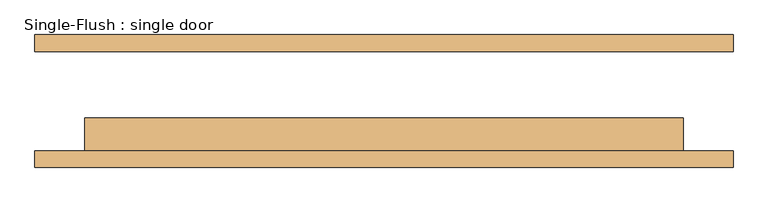
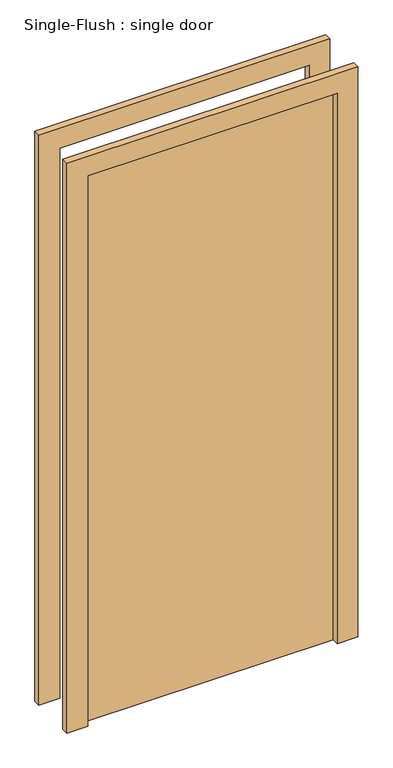
"""IFC4 building model written with IfcOpenShell, lengths in millimetres: door geometry, Single-Flush : single door."""

from ifc_helpers import new_model, si_unit, frame, origin, origin_with_axes, place, context, project, spatial, polyline, outline, extrude, source, transform, mapped, element, save


def single_flush_single_door_686f89d2(model_context):
    return source(origin(), model_context, "Body", "SweptSolid", [
        extrude(outline(polyline([(2209.8, -533.4), (0.0, -533.4), (0.0, -457.2), (2133.6, -457.2), (2133.6, 457.2), (0.0, 457.2), (0.0, 533.4), (2209.8, 533.4), (2209.8, -533.4)])), frame((0.0, -101.6, 0.0), z_axis=(0.0, 1.0, 0.0), x_axis=(0.0, 0.0, 1.0)), (0.0, 0.0, 1.0), 25.4),
        extrude(outline(polyline([(2209.8, 533.4), (2209.8, -533.4), (0.0, -533.4), (0.0, -457.2), (2133.6, -457.2), (2133.6, 457.2), (0.0, 457.2), (0.0, 533.4), (2209.8, 533.4)])), frame((0.0, 76.2, 0.0), z_axis=(0.0, 1.0, 0.0), x_axis=(0.0, 0.0, 1.0)), (0.0, 0.0, 1.0), 25.4),
        extrude(outline(polyline([(457.2, -25.4), (457.2, -76.2), (-457.2, -76.2), (-457.2, -25.4), (457.2, -25.4)])), origin_with_axes(), (0.0, 0.0, 1.0), 2133.6),
    ])


if __name__ == "__main__":
    model = new_model("IFC4")
    model_context = context("Model", 3, world=origin())
    ifc_project = project(units=[si_unit("LENGTHUNIT", "METRE", prefix="MILLI")], contexts=[model_context])
    site = spatial("IfcSite", under=ifc_project)
    building = spatial("IfcBuilding", under=site)
    placement = place(None, origin())
    single_flush_single_door_shape = single_flush_single_door_686f89d2(model_context)
    element("IfcDoor", 1, ObjectType="Single-Flush : single door", at=placement, inside=building, context=model_context, shape_type="MappedRepresentation", body=[
        mapped(single_flush_single_door_shape, transform((0.0, 0.0, 0.0), x_axis=(1.0, 0.0, 0.0), y_axis=(0.0, 1.0, 0.0), z_axis=(0.0, 0.0, 1.0))),
    ])
    save(model, "model.ifc")

# Revit data of these elements
# Type "Single-Flush : single door"
#   Type Mark = "11"
#   Construction Type Id = "MDOOR"
#   Assembly Code = "C1020"
#   Analytic Construction = "Metal"
#   Thickness = 0' - 2"
#   Heat Transfer Coefficient (U) = 0.651978 BTU/(h·ft²·°F)
#   Height = 7' - 0"
#   Trim Projection Ext = 0' - 1"
#   Trim Projection Int = 0' - 1"
#   Trim Width = 0' - 3"
#   Width = 3' - 0"
#   Define Thermal Properties by = 1
#   Door Material = Door - Panel
#   Frame Material = Door - Frame
#   Visual Light Transmittance = 0
#   Solar Heat Gain Coefficient = 0
#   Function = (empty or 0)
#   Wall Closure = (empty or 0)
# Element 1 (IfcDoor, "Single-Flush : single door")
#   Materials on its faces: "Door - Frame", "Door - Panel"
# Materials
#   "Door - Panel": class "Wood", colour RGB 210 159 95, transparency 0
#   "Door - Frame": colour RGB 118 70 51, transparency 0
